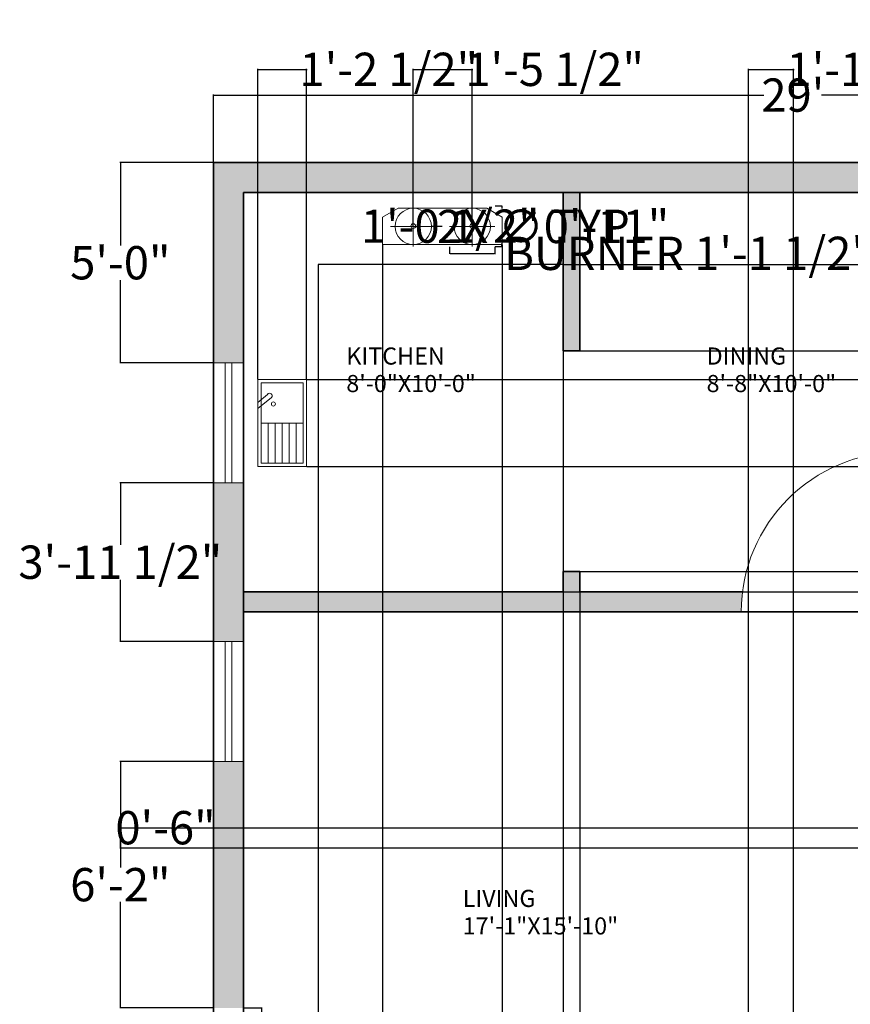
# Model space of a CAD drawing. Units: inches. Extents: x 2172 to 2712, y 1494 to 2108.
# Tile 2 of 3: x 2172 to 2422, y 1812 to 2108. Entities that reach past the tile are written whole.
import ezdxf

# ---------------------------------------------------------------- set-up
doc = ezdxf.new("R2010")
doc.units = ezdxf.units.IN
doc.header["$MEASUREMENT"] = 0
for name, color, linetype, lineweight in [('A-ANNO-DIMS', 2, 'Continuous', 18), ('A-AREA-IDEN', 7, 'Continuous', 18), ('A-DOOR', 3, 'Continuous', 18), ('A-EQPM', 8, 'Continuous', 18), ('A-FLOR-CASE', 9, 'Continuous', 25), ('A-FLOR-FIXT', 9, 'Continuous', 18), ('A-GLAZ', 4, 'Continuous', 18), ('A-WALL', 7, 'Continuous', 35)]:
    doc.layers.add(name, color=color, linetype=linetype, lineweight=lineweight)
doc.layers.add('A-WALL-PATT', color=251, linetype='Continuous', lineweight=13, true_color=0x636466)
doc.styles.get("Standard").update_dxf_attribs({"font": 'arial.ttf'})
doc.dimstyles.get("Standard").update_dxf_attribs({"dimtxt": 10, "dimasz": 0.18, "dimexe": 0.18, "dimexo": 0.0625, "dimgap": 0.09, "dimtad": 0, "dimtih": 1, "dimtoh": 1, "dimdec": 0, "dimzin": 0, "dimdsep": 46, "dimlunit": 3, "dimtxsty": 'Standard', "dimcen": 0.09, "dimadec": 0, "dimazin": 0, "dimtfac": 1, "dimtdec": 0, "dimtofl": 0, "dimtmove": 0, "dimatfit": 3, "dimfxl": 1, "dimtolj": 1, "dimtzin": 0, "dimarcsym": 0})

# ---------------------------------------------------------------- blocks, each defined once
blk = doc.blocks.new('*D3')
at = {"layer": 'A-ANNO-DIMS', "color": 0, "lineweight": -2, "transparency": 16777216}
for p, q in [((2230.53, 2064.8), (2230.53, 2085.18)), ((2230.71, 2085), (2395.86, 2085)), ((2578.35, 2085), (2413.19, 2085)), ((2578.53, 2064.8), (2578.53, 2085.18))]:
    blk.add_line(p, q, dxfattribs=at)
at = {"layer": 'A-ANNO-DIMS', "color": 0, "transparency": 16777216}
for points in [[(2230.71, 2085.03), (2230.71, 2084.97), (2230.53, 2085)], [(2578.35, 2085.03), (2578.35, 2084.97), (2578.53, 2085)]]:
    blk.add_solid(points, dxfattribs=at)
at = {"layer": 'Defpoints', "color": 0, "transparency": 16777216}
for p in [(2578.53, 2085), (2230.53, 2064.74), (2578.53, 2064.74)]:
    blk.add_point(p, dxfattribs=at)
at = {"layer": 'A-ANNO-DIMS', "color": 0, "transparency": 16777216, "insert": (2404.53, 2085), "char_height": 10, "attachment_point": 5}
blk.add_mtext("\\A1;29'", dxfattribs=at)
blk = doc.blocks.new('WIN-36IN')
for p, q in [((0, 36), (9, 36)), ((3.5, 36), (3.5, 0)), ((5.5, 36), (5.5, 0)), ((9, 0), (0, 0))]:
    blk.add_line(p, q)
blk = doc.blocks.new('DOOR-SWING-48IN')
for p, q in [((47, 0), (47, 48)), ((48, 0), (48, 48))]:
    blk.add_line(p, q)
blk.add_arc((48, 0), 48, 90, 180)
blk = doc.blocks.new('COOKTOP-BURNER')
for p, q in [((6.81, 12.26), (6.81, 0)), ((1.35, 6.05), (0, 6.05)), ((1.35, 6.05), (13.61, 6.05))]:
    blk.add_line(p, q)
for centre, radius in [((6.81, 6.05), 5.46), ((6.81, 6.13), 0.704)]:
    blk.add_circle(centre, radius)
blk = doc.blocks.new('*D9')
at = {"layer": 'A-ANNO-DIMS', "color": 0, "lineweight": -2, "transparency": 16777216}
for p, q in [((2239.59, 1810.79), (2245.11, 1810.79)), ((2244.93, 1810.61), (2244.93, 1798.06)), ((2244.93, 1774.97), (2244.93, 1787.53)), ((2239.59, 1774.79), (2245.11, 1774.79))]:
    blk.add_line(p, q, dxfattribs=at)
at = {"layer": 'A-ANNO-DIMS', "color": 0, "transparency": 16777216}
for points in [[(2244.9, 1810.61), (2244.96, 1810.61), (2244.93, 1810.79)], [(2244.9, 1774.97), (2244.96, 1774.97), (2244.93, 1774.79)]]:
    blk.add_solid(points, dxfattribs=at)
at = {"layer": 'Defpoints', "color": 0, "transparency": 16777216}
for p in [(2239.53, 1810.79), (2244.93, 1810.79), (2239.53, 1774.79)]:
    blk.add_point(p, dxfattribs=at)
at = {"layer": 'A-ANNO-DIMS', "color": 0, "transparency": 16777216, "insert": (2244.93, 1792.79), "char_height": 10, "attachment_point": 5}
blk.add_mtext('\\A1;WINDOW 3\'-0" TYP.', dxfattribs=at)
blk = doc.blocks.new('*D19')
at = {"layer": 'A-ANNO-DIMS', "color": 0, "lineweight": -2, "transparency": 16777216}
for p, q in [((2301.42, 2039.44), (2301.42, 2037.28)), ((2315.03, 2039.44), (2315.03, 2037.28)), ((2301.6, 2037.46), (2314.85, 2037.46)), ((2315.03, 2037.46), (2315.21, 2037.46))]:
    blk.add_line(p, q, dxfattribs=at)
at = {"layer": 'A-ANNO-DIMS', "color": 0, "transparency": 16777216}
for points in [[(2301.6, 2037.49), (2301.6, 2037.43), (2301.42, 2037.46)], [(2314.85, 2037.49), (2314.85, 2037.43), (2315.03, 2037.46)]]:
    blk.add_solid(points, dxfattribs=at)
at = {"layer": 'Defpoints', "color": 0, "transparency": 16777216}
for p in [(2301.42, 2039.5), (2315.03, 2039.5), (2315.03, 2037.46)]:
    blk.add_point(p, dxfattribs=at)
at = {"layer": 'A-ANNO-DIMS', "color": 0, "transparency": 16777216, "insert": (2388.65, 2037.46), "char_height": 10, "attachment_point": 5}
blk.add_mtext('\\A1;BURNER 1\'-1 1/2" TYP.', dxfattribs=at)
blk = doc.blocks.new('*D20')
at = {"layer": 'A-ANNO-DIMS', "color": 0, "lineweight": -2, "transparency": 16777216}
for p, q in [((2315.1, 2051.77), (2317.25, 2051.77)), ((2317.07, 2051.59), (2317.07, 2050.9)), ((2315.1, 2039.5), (2317.25, 2039.5)), ((2317.07, 2039.68), (2317.07, 2040.37))]:
    blk.add_line(p, q, dxfattribs=at)
at = {"layer": 'A-ANNO-DIMS', "color": 0, "transparency": 16777216}
for points in [[(2317.04, 2051.59), (2317.1, 2051.59), (2317.07, 2051.77)], [(2317.04, 2039.68), (2317.1, 2039.68), (2317.07, 2039.5)]]:
    blk.add_solid(points, dxfattribs=at)
at = {"layer": 'Defpoints', "color": 0, "transparency": 16777216}
for p in [(2315.03, 2051.77), (2317.07, 2051.77), (2315.03, 2039.5)]:
    blk.add_point(p, dxfattribs=at)
at = {"layer": 'A-ANNO-DIMS', "color": 0, "transparency": 16777216, "insert": (2317.07, 2045.63), "char_height": 10, "attachment_point": 5}
blk.add_mtext('\\A1;1\'-0 1/2" TYP.', dxfattribs=at)
blk = doc.blocks.new('*D21')
at = {"layer": 'A-ANNO-DIMS', "color": 0, "lineweight": -2, "transparency": 16777216}
for p, q in [((2230.46, 2064.74), (2202.35, 2064.74)), ((2202.53, 2064.56), (2202.53, 2039.83)), ((2202.53, 2004.71), (2202.53, 2029.44)), ((2230.46, 2004.53), (2202.35, 2004.53))]:
    blk.add_line(p, q, dxfattribs=at)
at = {"layer": 'A-ANNO-DIMS', "color": 0, "transparency": 16777216}
for points in [[(2202.5, 2064.56), (2202.56, 2064.56), (2202.53, 2064.74)], [(2202.5, 2004.71), (2202.56, 2004.71), (2202.53, 2004.53)]]:
    blk.add_solid(points, dxfattribs=at)
at = {"layer": 'Defpoints', "color": 0, "transparency": 16777216}
for p in [(2230.53, 2064.74), (2202.53, 2004.53), (2230.53, 2004.53)]:
    blk.add_point(p, dxfattribs=at)
at = {"layer": 'A-ANNO-DIMS', "color": 0, "transparency": 16777216, "insert": (2202.53, 2034.64), "char_height": 10, "attachment_point": 5}
blk.add_mtext('\\A1;5\'-0"', dxfattribs=at)
blk = doc.blocks.new('*D22')
at = {"layer": 'A-ANNO-DIMS', "color": 0, "lineweight": -2, "transparency": 16777216}
for p, q in [((2230.46, 1968.53), (2202.35, 1968.53)), ((2202.53, 1968.35), (2202.53, 1949.94)), ((2202.53, 1921), (2202.53, 1939.41)), ((2230.46, 1920.82), (2202.35, 1920.82))]:
    blk.add_line(p, q, dxfattribs=at)
at = {"layer": 'A-ANNO-DIMS', "color": 0, "transparency": 16777216}
for points in [[(2202.5, 1968.35), (2202.56, 1968.35), (2202.53, 1968.53)], [(2202.5, 1921), (2202.56, 1921), (2202.53, 1920.82)]]:
    blk.add_solid(points, dxfattribs=at)
at = {"layer": 'Defpoints', "color": 0, "transparency": 16777216}
for p in [(2230.53, 1968.53), (2202.53, 1920.82), (2230.53, 1920.82)]:
    blk.add_point(p, dxfattribs=at)
at = {"layer": 'A-ANNO-DIMS', "color": 0, "transparency": 16777216, "insert": (2202.53, 1944.68), "char_height": 10, "attachment_point": 5}
blk.add_mtext('\\A1;3\'-11 1/2"', dxfattribs=at)
blk = doc.blocks.new('*D23')
at = {"layer": 'A-ANNO-DIMS', "color": 0, "lineweight": -2, "transparency": 16777216}
for p, q in [((2230.46, 1884.82), (2202.35, 1884.82)), ((2202.53, 1884.64), (2202.53, 1853)), ((2202.53, 1810.97), (2202.53, 1842.61)), ((2230.46, 1810.79), (2202.35, 1810.79))]:
    blk.add_line(p, q, dxfattribs=at)
at = {"layer": 'A-ANNO-DIMS', "color": 0, "transparency": 16777216}
for points in [[(2202.5, 1884.64), (2202.56, 1884.64), (2202.53, 1884.82)], [(2202.5, 1810.97), (2202.56, 1810.97), (2202.53, 1810.79)]]:
    blk.add_solid(points, dxfattribs=at)
at = {"layer": 'Defpoints', "color": 0, "transparency": 16777216}
for p in [(2230.53, 1884.82), (2202.53, 1810.79), (2230.53, 1810.79)]:
    blk.add_point(p, dxfattribs=at)
at = {"layer": 'A-ANNO-DIMS', "color": 0, "transparency": 16777216, "insert": (2202.53, 1847.81), "char_height": 10, "attachment_point": 5}
blk.add_mtext('\\A1;6\'-2"', dxfattribs=at)
blk = doc.blocks.new('*D32')
at = {"layer": 'A-ANNO-DIMS', "color": 0, "lineweight": -2, "transparency": 16777216}
for p, q in [((2391.23, 1545.8), (2391.23, 2092.92)), ((2391.41, 2092.74), (2404.56, 2092.74)), ((2404.74, 1545.8), (2404.74, 2092.92)), ((2404.74, 2092.74), (2404.92, 2092.74))]:
    blk.add_line(p, q, dxfattribs=at)
at = {"layer": 'A-ANNO-DIMS', "color": 0, "transparency": 16777216}
for points in [[(2391.41, 2092.77), (2391.41, 2092.71), (2391.23, 2092.74)], [(2404.56, 2092.77), (2404.56, 2092.71), (2404.74, 2092.74)]]:
    blk.add_solid(points, dxfattribs=at)
at = {"layer": 'Defpoints', "color": 0, "transparency": 16777216}
for p in [(2404.74, 2092.74), (2391.23, 1545.74), (2404.74, 1545.74)]:
    blk.add_point(p, dxfattribs=at)
at = {"layer": 'A-ANNO-DIMS', "color": 0, "transparency": 16777216, "insert": (2429.48, 2092.74), "char_height": 10, "attachment_point": 5}
blk.add_mtext('\\A1;1\'-1 1/2"', dxfattribs=at)
blk = doc.blocks.new('*D34')
at = {"layer": 'A-ANNO-DIMS', "color": 0, "lineweight": -2, "transparency": 16777216}
for p, q in [((2239.53, 1935.68), (2239.53, 1508.56)), ((2261.99, 1935.68), (2261.99, 1508.56)), ((2239.71, 1508.74), (2261.81, 1508.74)), ((2261.99, 1508.74), (2262.17, 1508.74))]:
    blk.add_line(p, q, dxfattribs=at)
at = {"layer": 'A-ANNO-DIMS', "color": 0, "transparency": 16777216}
for points in [[(2239.71, 1508.77), (2239.71, 1508.71), (2239.53, 1508.74)], [(2261.81, 1508.77), (2261.81, 1508.71), (2261.99, 1508.74)]]:
    blk.add_solid(points, dxfattribs=at)
at = {"layer": 'Defpoints', "color": 0, "transparency": 16777216}
for p in [(2239.53, 1935.74), (2261.99, 1935.74), (2261.99, 1508.74)]:
    blk.add_point(p, dxfattribs=at)
at = {"layer": 'A-ANNO-DIMS', "color": 0, "transparency": 16777216, "insert": (2290.62, 1508.74), "char_height": 10, "attachment_point": 5}
blk.add_mtext('\\A1;1\'-10 1/2"', dxfattribs=at)
blk = doc.blocks.new('*D35')
at = {"layer": 'A-ANNO-DIMS', "color": 0, "lineweight": -2, "transparency": 16777216}
for p, q in [((2335.59, 2055.74), (2606.71, 2055.74)), ((2606.53, 2055.56), (2606.53, 2050.17)), ((2606.53, 2034.27), (2606.53, 2039.65)), ((2335.59, 2034.09), (2606.71, 2034.09))]:
    blk.add_line(p, q, dxfattribs=at)
at = {"layer": 'A-ANNO-DIMS', "color": 0, "transparency": 16777216}
for points in [[(2606.5, 2055.56), (2606.56, 2055.56), (2606.53, 2055.74)], [(2606.5, 2034.27), (2606.56, 2034.27), (2606.53, 2034.09)]]:
    blk.add_solid(points, dxfattribs=at)
at = {"layer": 'Defpoints', "color": 0, "transparency": 16777216}
for p in [(2335.53, 2055.74), (2335.53, 2034.09), (2606.53, 2034.09)]:
    blk.add_point(p, dxfattribs=at)
at = {"layer": 'A-ANNO-DIMS', "color": 0, "transparency": 16777216, "insert": (2606.53, 2044.91), "char_height": 10, "attachment_point": 5}
blk.add_mtext('\\A1;1\'-9 1/2"', dxfattribs=at)
blk = doc.blocks.new('*D36')
at = {"layer": 'A-ANNO-DIMS', "color": 0, "lineweight": -2, "transparency": 16777216}
for p, q in [((2243.82, 1999.66), (2243.82, 2092.92)), ((2244, 2092.74), (2258.26, 2092.74)), ((2258.44, 1999.66), (2258.44, 2092.92)), ((2258.44, 2092.74), (2258.62, 2092.74))]:
    blk.add_line(p, q, dxfattribs=at)
at = {"layer": 'A-ANNO-DIMS', "color": 0, "transparency": 16777216}
for points in [[(2244, 2092.77), (2244, 2092.71), (2243.82, 2092.74)], [(2258.26, 2092.77), (2258.26, 2092.71), (2258.44, 2092.74)]]:
    blk.add_solid(points, dxfattribs=at)
at = {"layer": 'Defpoints', "color": 0, "transparency": 16777216}
for p in [(2258.44, 2092.74), (2243.82, 1999.6), (2258.44, 1999.6)]:
    blk.add_point(p, dxfattribs=at)
at = {"layer": 'A-ANNO-DIMS', "color": 0, "transparency": 16777216, "insert": (2283.18, 2092.74), "char_height": 10, "attachment_point": 5}
blk.add_mtext('\\A1;1\'-2 1/2"', dxfattribs=at)
blk = doc.blocks.new('*D37')
at = {"layer": 'A-ANNO-DIMS', "color": 0, "lineweight": -2, "transparency": 16777216}
for p, q in [((2258.5, 1999.6), (2606.71, 1999.6)), ((2606.53, 1999.42), (2606.53, 1991.6)), ((2606.53, 1973.56), (2606.53, 1981.38)), ((2258.5, 1973.38), (2606.71, 1973.38))]:
    blk.add_line(p, q, dxfattribs=at)
at = {"layer": 'A-ANNO-DIMS', "color": 0, "transparency": 16777216}
for points in [[(2606.5, 1999.42), (2606.56, 1999.42), (2606.53, 1999.6)], [(2606.5, 1973.56), (2606.56, 1973.56), (2606.53, 1973.38)]]:
    blk.add_solid(points, dxfattribs=at)
at = {"layer": 'Defpoints', "color": 0, "transparency": 16777216}
for p in [(2258.44, 1999.6), (2258.44, 1973.38), (2606.53, 1973.38)]:
    blk.add_point(p, dxfattribs=at)
at = {"layer": 'A-ANNO-DIMS', "color": 0, "transparency": 16777216, "insert": (2606.53, 1986.49), "char_height": 10, "attachment_point": 5}
blk.add_mtext('\\A1;2\'-2"', dxfattribs=at)
blk = doc.blocks.new('*D38')
at = {"layer": 'A-ANNO-DIMS', "color": 0, "lineweight": -2, "transparency": 16777216}
for p, q in [((2335.59, 2008.15), (2606.71, 2008.15)), ((2606.53, 2007.97), (2606.53, 1980.23)), ((2606.53, 1942.09), (2606.53, 1969.84)), ((2335.59, 1941.91), (2606.71, 1941.91))]:
    blk.add_line(p, q, dxfattribs=at)
at = {"layer": 'A-ANNO-DIMS', "color": 0, "transparency": 16777216}
for points in [[(2606.5, 2007.97), (2606.56, 2007.97), (2606.53, 2008.15)], [(2606.5, 1942.09), (2606.56, 1942.09), (2606.53, 1941.91)]]:
    blk.add_solid(points, dxfattribs=at)
at = {"layer": 'Defpoints', "color": 0, "transparency": 16777216}
for p in [(2335.53, 2008.15), (2335.53, 1941.91), (2606.53, 1941.91)]:
    blk.add_point(p, dxfattribs=at)
at = {"layer": 'A-ANNO-DIMS', "color": 0, "transparency": 16777216, "insert": (2606.53, 1975.03), "char_height": 10, "attachment_point": 5}
blk.add_mtext('\\A1;5\'-6"', dxfattribs=at)
blk = doc.blocks.new('*D39')
at = {"layer": 'A-ANNO-DIMS', "color": 0, "lineweight": -2, "transparency": 16777216}
for p, q in [((2281.31, 2040.03), (2281.31, 1508.56)), ((2317.25, 2040.03), (2317.25, 1508.56)), ((2281.49, 1508.74), (2285.91, 1508.74)), ((2317.07, 1508.74), (2312.66, 1508.74))]:
    blk.add_line(p, q, dxfattribs=at)
at = {"layer": 'A-ANNO-DIMS', "color": 0, "transparency": 16777216}
for points in [[(2281.49, 1508.77), (2281.49, 1508.71), (2281.31, 1508.74)], [(2317.07, 1508.77), (2317.07, 1508.71), (2317.25, 1508.74)]]:
    blk.add_solid(points, dxfattribs=at)
at = {"layer": 'Defpoints', "color": 0, "transparency": 16777216}
for p in [(2281.31, 2040.1), (2317.25, 2040.1), (2317.25, 1508.74)]:
    blk.add_point(p, dxfattribs=at)
at = {"layer": 'A-ANNO-DIMS', "color": 0, "transparency": 16777216, "insert": (2299.28, 1508.74), "char_height": 10, "attachment_point": 5}
blk.add_mtext('\\A1;3\'-0"', dxfattribs=at)
blk = doc.blocks.new('*D40')
at = {"layer": 'A-ANNO-DIMS', "color": 0, "lineweight": -2, "transparency": 16777216}
for p, q in [((2290.5, 2045.62), (2290.5, 2092.92)), ((2290.68, 2092.74), (2308.05, 2092.74)), ((2308.23, 2045.62), (2308.23, 2092.92)), ((2308.23, 2092.74), (2308.41, 2092.74))]:
    blk.add_line(p, q, dxfattribs=at)
at = {"layer": 'A-ANNO-DIMS', "color": 0, "transparency": 16777216}
for points in [[(2290.68, 2092.77), (2290.68, 2092.71), (2290.5, 2092.74)], [(2308.05, 2092.77), (2308.05, 2092.71), (2308.23, 2092.74)]]:
    blk.add_solid(points, dxfattribs=at)
at = {"layer": 'Defpoints', "color": 0, "transparency": 16777216}
for p in [(2308.23, 2092.74), (2290.5, 2045.55), (2308.23, 2045.55)]:
    blk.add_point(p, dxfattribs=at)
at = {"layer": 'A-ANNO-DIMS', "color": 0, "transparency": 16777216, "insert": (2332.98, 2092.74), "char_height": 10, "attachment_point": 5}
blk.add_mtext('\\A1;1\'-5 1/2"', dxfattribs=at)
blk = doc.blocks.new('*D43')
at = {"layer": 'A-ANNO-DIMS', "color": 0, "lineweight": -2, "transparency": 16777216}
for p, q in [((2335.53, 1941.85), (2335.53, 1508.56)), ((2340.53, 1941.85), (2340.53, 1508.56)), ((2335.71, 1508.74), (2340.35, 1508.74)), ((2340.53, 1508.74), (2340.71, 1508.74))]:
    blk.add_line(p, q, dxfattribs=at)
at = {"layer": 'A-ANNO-DIMS', "color": 0, "transparency": 16777216}
for points in [[(2335.71, 1508.77), (2335.71, 1508.71), (2335.53, 1508.74)], [(2340.35, 1508.77), (2340.35, 1508.71), (2340.53, 1508.74)]]:
    blk.add_solid(points, dxfattribs=at)
at = {"layer": 'Defpoints', "color": 0, "transparency": 16777216}
for p in [(2335.53, 1941.91), (2340.53, 1941.91), (2340.53, 1508.74)]:
    blk.add_point(p, dxfattribs=at)
at = {"layer": 'A-ANNO-DIMS', "color": 0, "transparency": 16777216, "insert": (2354.09, 1508.74), "char_height": 10, "attachment_point": 5}
blk.add_mtext('\\A1;0\'-5"', dxfattribs=at)
blk = doc.blocks.new('*D44')
at = {"layer": 'A-ANNO-DIMS', "color": 0, "lineweight": -2, "transparency": 16777216}
for p, q in [((2494.46, 1864.74), (2202.35, 1864.74)), ((2202.53, 1864.74), (2202.53, 1864.92)), ((2202.53, 1864.92), (2202.71, 1864.92)), ((2202.53, 1858.92), (2202.53, 1864.56)), ((2488.46, 1858.74), (2202.35, 1858.74))]:
    blk.add_line(p, q, dxfattribs=at)
at = {"layer": 'A-ANNO-DIMS', "color": 0, "transparency": 16777216}
for points in [[(2202.5, 1864.56), (2202.56, 1864.56), (2202.53, 1864.74)], [(2202.5, 1858.92), (2202.56, 1858.92), (2202.53, 1858.74)]]:
    blk.add_solid(points, dxfattribs=at)
at = {"layer": 'Defpoints', "color": 0, "transparency": 16777216}
for p in [(2202.53, 1864.74), (2494.53, 1864.74), (2488.53, 1858.74)]:
    blk.add_point(p, dxfattribs=at)
at = {"layer": 'A-ANNO-DIMS', "color": 0, "transparency": 16777216, "insert": (2216.09, 1864.92), "char_height": 10, "attachment_point": 5}
blk.add_mtext('\\A1;0\'-6"', dxfattribs=at)
blk = doc.blocks.new('*D45')
at = {"layer": 'A-ANNO-DIMS', "color": 0, "lineweight": -2, "transparency": 16777216}
for p, q in [((2258.5, 1973.38), (2606.71, 1973.38)), ((2606.53, 1973.2), (2606.53, 1959.83)), ((2606.53, 1935.92), (2606.53, 1949.3)), ((2262.05, 1935.74), (2606.71, 1935.74))]:
    blk.add_line(p, q, dxfattribs=at)
at = {"layer": 'A-ANNO-DIMS', "color": 0, "transparency": 16777216}
for points in [[(2606.5, 1973.2), (2606.56, 1973.2), (2606.53, 1973.38)], [(2606.5, 1935.92), (2606.56, 1935.92), (2606.53, 1935.74)]]:
    blk.add_solid(points, dxfattribs=at)
at = {"layer": 'Defpoints', "color": 0, "transparency": 16777216}
for p in [(2258.44, 1973.38), (2261.99, 1935.74), (2606.53, 1935.74)]:
    blk.add_point(p, dxfattribs=at)
at = {"layer": 'A-ANNO-DIMS', "color": 0, "transparency": 16777216, "insert": (2606.53, 1954.56), "char_height": 10, "attachment_point": 5}
blk.add_mtext('\\A1;3\'-1 1/2"', dxfattribs=at)
blk = doc.blocks.new('*D46')
at = {"layer": 'A-ANNO-DIMS', "color": 0, "lineweight": -2, "transparency": 16777216}
for p, q in [((2317.25, 2040.03), (2317.25, 1508.56)), ((2335.53, 2034.02), (2335.53, 1508.56)), ((2317.43, 1508.74), (2335.35, 1508.74)), ((2335.53, 1508.74), (2335.71, 1508.74))]:
    blk.add_line(p, q, dxfattribs=at)
at = {"layer": 'A-ANNO-DIMS', "color": 0, "transparency": 16777216}
for points in [[(2317.43, 1508.77), (2317.43, 1508.71), (2317.25, 1508.74)], [(2335.35, 1508.77), (2335.35, 1508.71), (2335.53, 1508.74)]]:
    blk.add_solid(points, dxfattribs=at)
at = {"layer": 'Defpoints', "color": 0, "transparency": 16777216}
for p in [(2317.25, 2040.1), (2335.53, 2034.09), (2335.53, 1508.74)]:
    blk.add_point(p, dxfattribs=at)
at = {"layer": 'A-ANNO-DIMS', "color": 0, "transparency": 16777216, "insert": (2360.27, 1508.74), "char_height": 10, "attachment_point": 5}
blk.add_mtext('\\A1;1\'-6 1/2"', dxfattribs=at)
blk = doc.blocks.new('*D55')
at = {"layer": 'A-ANNO-DIMS', "color": 0, "lineweight": -2, "transparency": 16777216}
for p, q in [((2290.41, 2045.55), (2290.59, 2045.55)), ((2290.5, 2045.46), (2290.5, 2045.64)), ((2299.24, 2045.55), (2296.14, 2045.55))]:
    blk.add_line(p, q, dxfattribs=at)
at = {"layer": 'A-ANNO-DIMS', "color": 0, "transparency": 16777216}
blk.add_solid([(2296.14, 2045.58), (2296.14, 2045.52), (2295.96, 2045.55)], dxfattribs=at)
at = {"layer": 'Defpoints', "color": 0, "transparency": 16777216}
for p in [(2285.05, 2045.55), (2295.96, 2045.55)]:
    blk.add_point(p, dxfattribs=at)
at = {"layer": 'A-ANNO-DIMS', "color": 0, "transparency": 16777216, "insert": (2332.51, 2045.55), "char_height": 10, "attachment_point": 5}
blk.add_mtext('\\A1;2X ∅0\'-11"', dxfattribs=at)

msp = doc.modelspace()

# ---------------------------------------------------------------- hatches: boundary and pattern name
at = {"layer": 'A-WALL-PATT'}
h = msp.add_hatch(color=256, dxfattribs=at)
h.dxf.hatch_style = 1
h.paths.add_polyline_path([(2239.53, 1774.79), (2230.53, 1774.79), (2230.53, 1536.74), (2245.63, 1536.74), (2245.63, 1541.24), (2239.53, 1541.24)])
h.paths.add_polyline_path([(2569.53, 1545.74), (2379.53, 1545.74), (2379.53, 1536.74), (2569.53, 1536.74)])
h.paths.add_polyline_path([(2379.53, 1541.24), (2344.11, 1541.24), (2344.11, 1536.74), (2379.3, 1536.74)])
h.paths.add_polyline_path([(2578.53, 1561.68), (2569.53, 1561.68), (2569.53, 1536.74), (2578.53, 1536.74)])
h.paths.add_polyline_path([(2578.53, 1628.83), (2569.53, 1628.83), (2569.53, 1618.74), (2569.53, 1597.68), (2578.53, 1597.68)])
h.paths.add_polyline_path([(2578.53, 1721.29), (2569.53, 1721.29), (2569.53, 1672.74), (2569.53, 1656.53), (2578.53, 1656.53)])
h.paths.add_polyline_path([(2569.53, 1672.74), (2479.6, 1672.74, -0.062096), (2478.72, 1666.74), (2569.53, 1666.74)], flags=17)
h.paths.add_polyline_path([(2569.53, 1618.74), (2449.53, 1618.74), (2449.53, 1666.74), (2454.6, 1666.74), (2454.6, 1672.74), (2449.53, 1672.74), (2449.53, 1804.74), (2453.65, 1804.74), (2453.65, 1810.74), (2444.53, 1810.74), (2444.53, 1739.74), (2436.58, 1739.74), (2436.58, 1730.74), (2444.53, 1730.74), (2444.53, 1612.74), (2569.53, 1612.74)])
h.paths.add_polyline_path([(2384.53, 1730.74), (2379.53, 1730.74), (2379.53, 1612.74), (2384.53, 1612.74)])
h.paths.add_polyline_path([(2389.43, 1739.74), (2239.53, 1739.74), (2239.53, 1730.74), (2388.58, 1730.74, -0.047189)])
h.paths.add_polyline_path([(2569.53, 1810.74), (2494.53, 1810.74), (2494.53, 1832.1, -0.067617), (2488.53, 1831.74), (2488.53, 1830), (2488.53, 1804.74), (2569.53, 1804.74)])
h.paths.add_polyline_path([(2488.53, 1810.74), (2478.65, 1810.74, -0.063254), (2477.89, 1804.74), (2488.53, 1804.74)])
h.paths.add_polyline_path([(2569.53, 1864.74), (2488.53, 1864.74), (2488.53, 1858.74), (2569.53, 1858.74)])
h.paths.add_polyline_path([(2494.53, 1858.74), (2488.53, 1858.74), (2488.53, 1855), (2494.53, 1855)])
h.paths.add_polyline_path([(2494.53, 1887.05, -0.073561), (2488.53, 1888.74), (2488.53, 1885.18), (2488.53, 1879.18), (2488.53, 1864.74), (2494.53, 1864.74)])
h.paths.add_polyline_path([(2488.53, 1864.74), (2476.91, 1864.74, -0.063254), (2477.67, 1858.74), (2488.53, 1858.74)])
h.paths.add_polyline_path([(2449.53, 1918.74), (2449.53, 2055.74), (2444.53, 2055.74), (2444.53, 1912.74), (2444.53, 1858.74), (2449.53, 1858.74), (2452.67, 1858.74), (2452.67, 1864.74), (2449.53, 1864.74)])
h.paths.add_polyline_path([(2578.53, 1965.71), (2569.53, 1965.71), (2569.53, 1918.74), (2569.53, 1899.23), (2578.53, 1899.23)])
h.paths.add_polyline_path([(2578.53, 1825.85), (2569.53, 1825.85), (2569.53, 1757.29), (2578.53, 1757.29)])
h.paths.add_polyline_path([(2578.53, 1871.54), (2569.53, 1871.54), (2569.53, 1864.74), (2569.53, 1853.54), (2578.53, 1853.54)])
h.paths.add_polyline_path([(2239.53, 1884.82), (2230.53, 1884.82), (2230.53, 1810.79), (2239.53, 1810.79)])
h.paths.add_polyline_path([(2239.53, 1968.53), (2230.53, 1968.53), (2230.53, 1920.82), (2239.53, 1920.82), (2239.53, 1929.74)])
h.paths.add_polyline_path([(2389.42, 1935.74), (2340.53, 1935.74), (2340.53, 1941.91), (2335.53, 1941.91), (2335.53, 1935.74), (2239.53, 1935.74), (2239.53, 1929.74), (2340.53, 1929.74), (2389.05, 1929.74, -0.031342)])
h.paths.add_polyline_path([(2239.53, 2055.74), (2569.53, 2055.74), (2569.53, 2001.71), (2578.53, 2001.71), (2578.53, 2064.74), (2230.53, 2064.74), (2230.53, 2004.53), (2239.53, 2004.53)])
h.paths.add_polyline_path([(2340.53, 2055.74), (2335.53, 2055.74), (2335.53, 2008.15), (2340.53, 2008.15)], flags=17)
h.paths.add_polyline_path([(2444.53, 1935.74), (2437.05, 1935.74), (2437.05, 1929.74), (2444.53, 1929.74)])
h.paths.add_polyline_path([(2569.53, 1918.74), (2488.53, 1918.74), (2488.53, 1909.18), (2494.53, 1909.18), (2494.53, 1912.74), (2569.53, 1912.74)])

# ---------------------------------------------------------------- linework, layer by layer
at = {"layer": 'A-EQPM'}
for p, q in [((2281.31, 2048.32), (2285.98, 2051.01)), ((2285.98, 2051.01), (2312.58, 2051.01)), ((2317.25, 2048.32), (2312.58, 2051.01)), ((2281.31, 2048.32), (2281.31, 2040.1)), ((2317.25, 2040.1), (2317.25, 2048.32)), ((2281.31, 2040.1), (2317.25, 2040.1))]:
    msp.add_line(p, q, dxfattribs=at)
at = {"layer": 'A-FLOR-CASE'}
for p, q in [((2335.53, 2034.09), (2261.99, 2034.09)), ((2261.99, 2034.09), (2261.99, 1935.74))]:
    msp.add_line(p, q, dxfattribs=at)
at = {"layer": 'A-FLOR-FIXT'}
for p, q in [((2243.82, 1992.7), (2246.73, 1995.1)), ((2243.82, 1990.87), (2247.98, 1994.19)), ((2257.44, 1986.49), (2244.82, 1986.49)), ((2244.82, 1986.49), (2244.82, 1974.38)), ((2246.93, 1986.49), (2246.93, 1974.38)), ((2249.03, 1986.49), (2249.03, 1974.38)), ((2251.13, 1986.49), (2257.44, 1986.49)), ((2251.13, 1986.49), (2251.13, 1974.38)), ((2253.23, 1986.49), (2253.23, 1974.38)), ((2255.34, 1986.49), (2255.34, 1974.38)), ((2257.44, 1986.49), (2257.44, 1974.38))]:
    msp.add_line(p, q, dxfattribs=at)
for points in [[(2243.82, 1999.6), (2258.44, 1999.6), (2258.44, 1973.38), (2243.82, 1973.38)], [(2244.82, 1998.6), (2257.44, 1998.6), (2257.44, 1974.38), (2244.82, 1974.38)]]:
    msp.add_lwpolyline(points, close=True, dxfattribs=at)
msp.add_circle((2248.5, 1992.21), 0.613, dxfattribs=at)
msp.add_arc((2247.35, 1994.65), 0.772, 323.7789, 143.7789, dxfattribs=at)
at = {"layer": 'A-WALL'}
for p, q in [((2230.53, 2064.74), (2578.53, 2064.74)), ((2230.53, 2064.74), (2230.53, 1536.74)), ((2239.53, 2055.74), (2569.53, 2055.74)), ((2239.53, 2055.74), (2239.53, 1541.24)), ((2335.53, 2008.15), (2335.53, 2055.74)), ((2340.53, 2008.15), (2340.53, 2055.74)), ((2340.53, 2008.15), (2335.53, 2008.15)), ((2335.53, 1935.74), (2335.53, 1941.91)), ((2335.53, 1941.91), (2340.53, 1941.91)), ((2340.53, 1935.74), (2340.53, 1941.91)), ((2335.53, 1935.74), (2239.53, 1935.74)), ((2389.42, 1935.74), (2340.53, 1935.74)), ((2340.53, 1929.74), (2239.53, 1929.74)), ((2239.53, 1929.74), (2239.53, 1739.74)), ((2444.53, 1929.74), (2335.53, 1929.74))]:
    msp.add_line(p, q, dxfattribs=at)

# ---------------------------------------------------------------- block references
at = {"layer": 'A-DOOR'}
msp.add_blockref('DOOR-SWING-48IN', (2389.05, 1929.74), dxfattribs=at)
at = {"layer": 'A-EQPM'}
for p in [(2283.69, 2039.5), (2301.42, 2039.5)]:
    msp.add_blockref('COOKTOP-BURNER', p, dxfattribs=at)
at = {"layer": 'A-GLAZ'}
for p in [(2230.53, 1968.53), (2230.53, 1884.82)]:
    msp.add_blockref('WIN-36IN', p, dxfattribs=at)

# ---------------------------------------------------------------- texts
at = {"layer": 'A-AREA-IDEN'}
for s, height, p in [('KITCHEN', 5.144, (2270.4, 2004.04)), ('DINING', 5.144, (2378.62, 2004.04)), ('8\'-0"X10\'-0"', 5.1443, (2270.4, 1995.78)), ('8\'-8"X10\'-0"', 5.1443, (2378.62, 1995.78)), ('LIVING', 5.144, (2305.36, 1841.11)), ('17\'-1"X15\'-10"', 5.1443, (2305.36, 1832.84))]:
    msp.add_text(s, height=height, dxfattribs=at).set_placement(p)

# ---------------------------------------------------------------- dimensions: what is measured, and where the dimension line sits
at = {"layer": 'A-ANNO-DIMS'}
for base, p1, p2, override, picture, middle in [((2258.44, 2092.74), (2243.82, 1999.6), (2258.44, 1999.6), {"dimdec": 1, "dimlfac": 1, "dimrnd": 0, "dimzin": 1, "dimdsep": 46, "dimlunit": 4, "dimfrac": 2}, '*D36', (2283.18, 2092.74)), ((2308.23, 2092.74), (2290.5, 2045.55), (2308.23, 2045.55), {"dimdec": 1, "dimlfac": 1, "dimrnd": 0, "dimzin": 1, "dimdsep": 46, "dimlunit": 4, "dimfrac": 2}, '*D40', (2332.98, 2092.74)), ((2404.74, 2092.74), (2391.23, 1545.74), (2404.74, 1545.74), {"dimdec": 1, "dimlfac": 1, "dimrnd": 0, "dimzin": 1, "dimdsep": 46, "dimlunit": 4, "dimfrac": 2}, '*D32', (2429.48, 2092.74)), ((2578.53, 2085), (2230.53, 2064.74), (2578.53, 2064.74), {"dimclrd": 0, "dimclre": 0, "dimclrt": 0}, '*D3', (2404.53, 2085)), ((2317.25, 1508.74), (2281.31, 2040.1), (2317.25, 2040.1), {"dimdec": 1, "dimlfac": 1, "dimrnd": 0, "dimzin": 1, "dimdsep": 46, "dimlunit": 4, "dimfrac": 2}, '*D39', (2299.28, 1508.74)), ((2335.53, 1508.74), (2317.25, 2040.1), (2335.53, 2034.09), {"dimdec": 1, "dimlfac": 1, "dimrnd": 0, "dimzin": 1, "dimdsep": 46, "dimlunit": 4, "dimfrac": 2}, '*D46', (2360.27, 1508.74)), ((2340.53, 1508.74), (2335.53, 1941.91), (2340.53, 1941.91), {"dimdec": 1, "dimlfac": 1, "dimrnd": 0, "dimzin": 1, "dimdsep": 46, "dimlunit": 4, "dimfrac": 2}, '*D43', (2354.09, 1508.74)), ((2261.99, 1508.74), (2239.53, 1935.74), (2261.99, 1935.74), {"dimdec": 1, "dimlfac": 1, "dimrnd": 0, "dimzin": 1, "dimdsep": 46, "dimlunit": 4, "dimfrac": 2}, '*D34', (2290.62, 1508.74))]:
    dim = msp.add_linear_dim(base=base, p1=p1, p2=p2, dimstyle='Standard', override=override, dxfattribs=at)
    dim.commit()
    dim.dimension.update_dxf_attribs({"geometry": picture, "text_midpoint": middle})
for base, p1, p2, text, picture, middle in [((2317.07, 2051.77), (2315.03, 2039.5), (2315.03, 2051.77), '<> TYP.', '*D20', (2317.07, 2045.63)), ((2244.93, 1810.79), (2239.53, 1774.79), (2239.53, 1810.79), 'WINDOW <> TYP.', '*D9', (2244.93, 1792.79))]:
    dim = msp.add_linear_dim(base=base, p1=p1, p2=p2, angle=90, text=text, dimstyle='Standard', override={"dimdec": 1, "dimlfac": 1, "dimrnd": 0, "dimzin": 1, "dimdsep": 46, "dimlunit": 4, "dimfrac": 2}, dxfattribs=at)
    dim.commit()
    dim.dimension.update_dxf_attribs({"geometry": picture, "text_midpoint": middle})
dim = msp.add_linear_dim(base=(2315.03, 2037.46), p1=(2301.42, 2039.5), p2=(2315.03, 2039.5), text='BURNER <> TYP.', dimstyle='Standard', override={"dimdec": 1, "dimlfac": 1, "dimrnd": 0, "dimzin": 1, "dimdsep": 46, "dimlunit": 4, "dimfrac": 2}, dxfattribs=at)
dim.commit()
dim.dimension.update_dxf_attribs({"geometry": '*D19', "text_midpoint": (2388.65, 2037.46)})
for base, p1, p2, picture, middle in [((2202.53, 2004.53), (2230.53, 2064.74), (2230.53, 2004.53), '*D21', (2202.53, 2034.64)), ((2606.5253, 2034.0872), (2335.5253, 2055.7407), (2335.5253, 2034.0872), '*D35', (2606.5253, 2044.914)), ((2606.53, 1941.91), (2335.53, 2008.15), (2335.53, 1941.91), '*D38', (2606.53, 1975.03)), ((2606.53, 1973.38), (2258.44, 1999.6), (2258.44, 1973.38), '*D37', (2606.53, 1986.49)), ((2606.53, 1935.74), (2258.44, 1973.38), (2261.99, 1935.74), '*D45', (2606.53, 1954.56)), ((2202.53, 1920.82), (2230.53, 1968.53), (2230.53, 1920.82), '*D22', (2202.53, 1944.68)), ((2202.53, 1810.79), (2230.53, 1884.82), (2230.53, 1810.79), '*D23', (2202.53, 1847.81)), ((2202.53, 1864.74), (2488.53, 1858.74), (2494.53, 1864.74), '*D44', (2216.09, 1864.92))]:
    dim = msp.add_linear_dim(base=base, p1=p1, p2=p2, angle=90, dimstyle='Standard', override={"dimdec": 1, "dimlfac": 1, "dimrnd": 0, "dimzin": 1, "dimdsep": 46, "dimlunit": 4, "dimfrac": 2}, dxfattribs=at)
    dim.commit()
    dim.dimension.update_dxf_attribs({"geometry": picture, "text_midpoint": middle})
dim = msp.add_diameter_dim_2p(p1=(2285.05, 2045.55), p2=(2295.96, 2045.55), text='2X <>', dimstyle='Standard', override={"dimdec": 1, "dimlfac": 1, "dimrnd": 0, "dimzin": 1, "dimdsep": 46, "dimlunit": 4, "dimfrac": 2}, dxfattribs=at)
dim.commit()
dim.dimension.update_dxf_attribs({"geometry": '*D55', "text_midpoint": (2299.24, 2045.55), "dimtype": 163})

doc.saveas('drawing.dxf')
